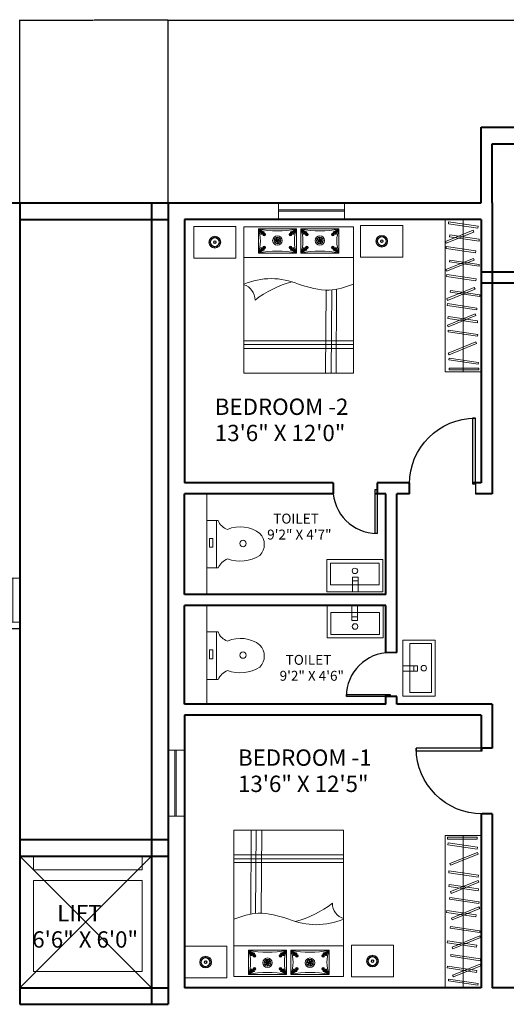
# Model space of a CAD drawing. Units: inches. Extents: x -46 to 1145, y -527 to 760.
# Tile 54 of 57: x 509 to 775, y 222 to 760. Entities that reach past the tile are written whole.
import ezdxf

# ---------------------------------------------------------------- set-up
doc = ezdxf.new("R2010")
doc.units = ezdxf.units.IN
doc.header["$MEASUREMENT"] = 0
for name, color, linetype, lineweight in [('A-ANNO-DIMS', 2, 'Continuous', 18), ('A-AREA-IDEN', 1, 'Continuous', 18), ('A-FLOR-CASE', 32, 'Continuous', 18), ('A-FLOR-EVTR', 6, 'Continuous', 18), ('A-FLOR-FIXT', 9, 'Continuous', 18), ('A-FURN', 2, 'Continuous', 13), ('DOORS', 3, 'Continuous', 25), ('WALLS', 4, 'Continuous', 40), ('WINDOWS', 240, 'Continuous', 20)]:
    doc.layers.add(name, color=color, linetype=linetype, lineweight=lineweight)
doc.layers.add('FURNTIURE', color=2, linetype='Continuous')
doc.layers.add('LT', color=9, linetype='Continuous')
doc.styles.get("Standard").update_dxf_attribs({"font": 'arial.ttf'})
doc.dimstyles.get("Standard").update_dxf_attribs({"dimtxt": 0.18, "dimasz": 0.18, "dimexe": 0.18, "dimexo": 0.0625, "dimgap": 0.09, "dimtad": 0, "dimtih": 1, "dimtoh": 1, "dimdec": 0, "dimzin": 0, "dimdsep": 46, "dimlunit": 3, "dimtxsty": 'Standard', "dimcen": 0.09, "dimadec": 0, "dimazin": 0, "dimtfac": 1, "dimtdec": 0, "dimtofl": 0, "dimtmove": 0, "dimatfit": 3, "dimfxl": 1, "dimtolj": 1, "dimtzin": 0, "dimarcsym": 0})

# ---------------------------------------------------------------- blocks, each defined once
blk = doc.blocks.new('*U2')
for p, q in [((0, 0), (0, -6)), ((40, 0), (40, -6))]:
    blk.add_line(p, q)
blk.add_lwpolyline([(0, 0), (0, 40), (1.75, 40), (1.75, 0)], close=True)
blk.add_arc((0, 0), 40, 0, 90)
blk = doc.blocks.new('*U89')
at = {"layer": 'FURNTIURE'}
blk.add_line((0, 0.42), (0, -0.42), dxfattribs=at)
blk = doc.blocks.new('*U90')
at = {"layer": 'FURNTIURE', "transparency": 16777216}
for p, rotation in [((589.5, 506.39), 54), ((590.11, 507), 36), ((590.89, 507.4), 17.99999999999997), ((592.61, 507.4), 341.9999999999999), ((593.39, 507), 324), ((594.01, 506.39), 306), ((588.97, 504.75), 90), ((589.1, 505.61), 72), ((589.1, 503.89), 108), ((589.5, 503.11), 126), ((590.11, 502.49), 144), ((590.89, 502.1), 162), ((591.75, 501.96), 180), ((592.61, 502.1), 197.9999999999999), ((593.39, 502.49), 216), ((594.01, 503.11), 234), ((594.4, 505.61), 288), ((594.4, 503.89), 252), ((594.54, 504.75), 270)]:
    blk.add_blockref('*U89', p, dxfattribs=dict(at, rotation=rotation))
blk.add_blockref('*U89', (591.75, 507.53), dxfattribs=at)
blk = doc.blocks.new('*U87')
at = {"layer": 'FURNTIURE'}
blk.add_line((0, 0.1), (0, -0.1), dxfattribs=at)
blk = doc.blocks.new('*U88')
at = {"layer": 'FURNTIURE', "transparency": 16777216}
for p, rotation in [((141.23, 121.04), 90), ((141.27, 121.25), 72), ((141.27, 120.83), 108), ((141.36, 121.43), 54), ((141.36, 120.65), 126), ((141.51, 121.58), 35.99999999999999), ((141.51, 120.5), 144), ((141.7, 121.67), 17.99999999999998), ((141.7, 120.4), 162), ((141.9, 120.37), 180), ((142.11, 121.67), 342), ((142.11, 120.4), 198), ((142.3, 121.58), 324), ((142.3, 120.5), 216), ((142.44, 121.43), 306), ((142.44, 120.65), 234), ((142.54, 121.25), 288), ((142.54, 120.83), 252), ((142.57, 121.04), 270)]:
    blk.add_blockref('*U87', p, dxfattribs=dict(at, rotation=rotation))
blk.add_blockref('*U87', (141.9, 121.71), dxfattribs=at)
blk = doc.blocks.new('NIGHTSTAND')
blk.add_lwpolyline([(23.06, 0), (0, 0), (0, 17.28), (23.06, 17.28)], close=True)
for radius in [3.21, 2.36, 0.77, 0.567]:
    blk.add_circle((11.53, 8.64), radius)
for name, p in [('*U90', (-580.22, -496.1)), ('*U88', (-130.37, -112.4))]:
    blk.add_blockref(name, p)
blk = doc.blocks.new('WARDROBE')
blk.add_line((9.78, 0), (9.78, 83.25))
for points in [[(19.56, 0), (0, 0), (0, 83.25), (19.56, 83.25)], [(17.74, 78.49), (1.66, 80.88), (1.8, 81.87), (17.88, 79.48)], [(15.55, 76.35), (0.49, 70.23), (0.11, 71.16), (15.17, 77.28)], [(18.43, 71.4), (2.35, 73.79), (2.5, 74.78), (18.58, 72.39)], [(16.47, 65.03), (0.39, 67.42), (0.54, 68.41), (16.62, 66.02)], [(15.79, 61), (0.73, 54.88), (0.35, 55.81), (15.41, 61.93)], [(18.43, 57.62), (2.35, 60.01), (2.5, 61), (18.58, 58.61)], [(16.71, 49.68), (0.63, 52.07), (0.78, 53.06), (16.86, 50.67)], [(16.22, 45.12), (1.16, 39), (0.78, 39.93), (15.84, 46.05)], [(18.77, 41.02), (2.69, 43.41), (2.84, 44.4), (18.92, 42.01)], [(17.14, 33.8), (1.06, 36.19), (1.21, 37.19), (17.29, 34.8)], [(16.65, 30.67), (1.59, 24.55), (1.21, 25.48), (16.27, 31.6)], [(17.52, 26.78), (1.44, 29.17), (1.59, 30.16), (17.67, 27.77)], [(17.57, 19.35), (1.49, 21.74), (1.64, 22.73), (17.72, 20.34)], [(17.08, 15.35), (2.02, 9.23), (1.64, 10.16), (16.7, 16.28)], [(18, 4.03), (1.92, 6.42), (2.07, 7.41), (18.15, 5.03)], [(18.32, 0.98), (2.07, 0.98), (2.07, 1.98), (18.32, 1.98)]]:
    blk.add_lwpolyline(points, close=True)
blk = doc.blocks.new('LAVATORY-RECT')
blk.add_line((14.01, 6.17), (17.08, 6.17))
for points in [[(30.61, 0), (0, 0), (0, 17.7), (30.61, 17.7)], [(28.7, 3.94), (1.97, 3.94), (1.97, 15.81), (28.7, 15.81)], [(17.08, 0), (14.01, 0), (14.01, 8.17), (17.08, 8.17)]]:
    blk.add_lwpolyline(points, close=True)
blk.add_circle((15.39, 11.51), 1.51)
blk = doc.blocks.new('WATER-CLOSET')
for p, q in [((0, 0), (0, 26.01)), ((0, 26.01), (6.13, 26.01)), ((5.22, 21.04), (5.22, 26.01)), ((5.22, 26.01), (5.22, 0)), ((0, 0), (6.13, 0))]:
    blk.add_line(p, q)
blk.add_lwpolyline([(1.51, 11.4), (1.51, 16.16), (3.34, 16.16), (3.34, 11.4)], close=True)
blk.add_circle((19.79, 13.37), 1.75)
for centre, radius, start, end in [((14.15, 29.2), 8.64, 201.6782, 251.0259), ((18.35, 4.96), 17.54, 52.4616, 113.5359), ((22.52, 12.84), 8.87, 317.2682, 42.7318), ((18.33, 23.71), 20, 249.5645, 302.3709), ((15.4, -4.5), 10.31, 113.1704, 154.0947)]:
    blk.add_arc(centre, radius, start, end)
blk = doc.blocks.new('WINDOW-36IN')
for p, q in [((0, 4.5), (0, 9)), ((0, 9), (0, 0)), ((36, 9), (36, 0)), ((0, 5.23), (36, 5.23)), ((0, 4.5), (36, 4.5))]:
    blk.add_line(p, q)
blk = doc.blocks.new('WINDOW-24IN')
for p, q in [((0, 4.5), (0, 9)), ((0, 9), (0, 0)), ((24, 9), (24, 0)), ((0, 5.23), (24, 5.23)), ((0, 4.5), (24, 4.5))]:
    blk.add_line(p, q)
blk = doc.blocks.new('*U58')
at = {"layer": 'LT'}
blk.add_line((0, 0.28), (0, -0.28), dxfattribs=at)
for centre, start, end in [((0.73, 0), 159.0676, 200.9324), ((-0.73, 0), 339.0676, 20.9324)]:
    blk.add_arc(centre, 0.786, start, end, dxfattribs=at)
blk = doc.blocks.new('*U59')
at = {"layer": 'LT', "transparency": 16777216}
for p, rotation in [((609.66, 443.79), 80.00000000000001), ((609.69, 443.6), 120), ((609.76, 443.96), 40.00000000000002), ((609.84, 443.48), 160), ((610.03, 443.48), 200), ((610.12, 443.96), 320), ((610.18, 443.6), 240), ((610.21, 443.79), 280)]:
    blk.add_blockref('*U58', p, dxfattribs=dict(at, rotation=rotation))
blk.add_blockref('*U58', (609.94, 444.03), dxfattribs=at)
blk = doc.blocks.new('*U60')
at = {"layer": 'LT'}
blk.add_line((0, 0.12), (0, -0.12), dxfattribs=at)
for centre, start, end in [((0.31, 0), 159.0676, 200.9324), ((-0.31, 0), 339.0676, 20.9324)]:
    blk.add_arc(centre, 0.335, start, end, dxfattribs=at)
blk = doc.blocks.new('*U61')
at = {"layer": 'LT', "transparency": 16777216}
for p, rotation in [((259.5, 188.9), 80.00000000000001), ((259.51, 188.82), 120), ((259.54, 188.97), 40), ((259.57, 188.76), 160), ((259.65, 188.76), 200), ((259.69, 188.97), 320), ((259.72, 188.82), 240), ((259.73, 188.9), 280)]:
    blk.add_blockref('*U60', p, dxfattribs=dict(at, rotation=rotation))
blk.add_blockref('*U60', (259.61, 189), dxfattribs=at)
blk = doc.blocks.new('*U62')
at = {"layer": 'LT'}
blk.add_line((0, 0.12), (0, -0.12), dxfattribs=at)
for centre, start, end in [((0.31, 0), 159.0676, 200.9324), ((-0.31, 0), 339.0676, 20.9324)]:
    blk.add_arc(centre, 0.335, start, end, dxfattribs=at)
blk = doc.blocks.new('*U63')
at = {"layer": 'LT', "transparency": 16777216}
for p, rotation in [((259.5, 188.9), 80.00000000000001), ((259.51, 188.82), 120), ((259.54, 188.97), 40), ((259.57, 188.76), 160), ((259.65, 188.76), 200), ((259.69, 188.97), 320), ((259.72, 188.82), 240), ((259.73, 188.9), 280)]:
    blk.add_blockref('*U62', p, dxfattribs=dict(at, rotation=rotation))
blk.add_blockref('*U62', (259.61, 189), dxfattribs=at)
blk = doc.blocks.new('*U64')
at = {"layer": 'LT'}
blk.add_line((0, 0.28), (0, -0.28), dxfattribs=at)
for centre, start, end in [((0.73, 0), 159.0676, 200.9324), ((-0.73, 0), 339.0676, 20.9324)]:
    blk.add_arc(centre, 0.786, start, end, dxfattribs=at)
blk = doc.blocks.new('*U65')
at = {"layer": 'LT', "transparency": 16777216}
for p, rotation in [((609.66, 443.79), 80.00000000000001), ((609.69, 443.6), 120), ((609.76, 443.96), 40.00000000000002), ((609.84, 443.48), 160), ((610.03, 443.48), 200), ((610.12, 443.96), 320), ((610.18, 443.6), 240), ((610.21, 443.79), 280)]:
    blk.add_blockref('*U64', p, dxfattribs=dict(at, rotation=rotation))
blk.add_blockref('*U64', (609.94, 444.03), dxfattribs=at)
blk = doc.blocks.new('*U66')
at = {"layer": 'LT'}
blk.add_line((0, 0.12), (0, -0.12), dxfattribs=at)
for centre, start, end in [((0.31, 0), 159.0676, 200.9324), ((-0.31, 0), 339.0676, 20.9324)]:
    blk.add_arc(centre, 0.335, start, end, dxfattribs=at)
blk = doc.blocks.new('*U67')
at = {"layer": 'LT', "transparency": 16777216}
for p, rotation in [((259.5, 188.9), 80.00000000000001), ((259.51, 188.82), 120), ((259.54, 188.97), 40), ((259.57, 188.76), 160), ((259.65, 188.76), 200), ((259.69, 188.97), 320), ((259.72, 188.82), 240), ((259.73, 188.9), 280)]:
    blk.add_blockref('*U66', p, dxfattribs=dict(at, rotation=rotation))
blk.add_blockref('*U66', (259.61, 189), dxfattribs=at)
blk = doc.blocks.new('*U68')
at = {"layer": 'LT'}
blk.add_line((0, 0.12), (0, -0.12), dxfattribs=at)
for centre, start, end in [((0.31, 0), 159.0676, 200.9324), ((-0.31, 0), 339.0676, 20.9324)]:
    blk.add_arc(centre, 0.335, start, end, dxfattribs=at)
blk = doc.blocks.new('*U69')
at = {"layer": 'LT', "transparency": 16777216}
for p, rotation in [((259.5, 188.9), 80.00000000000001), ((259.51, 188.82), 120), ((259.54, 188.97), 40), ((259.57, 188.76), 160), ((259.65, 188.76), 200), ((259.69, 188.97), 320), ((259.72, 188.82), 240), ((259.73, 188.9), 280)]:
    blk.add_blockref('*U68', p, dxfattribs=dict(at, rotation=rotation))
blk.add_blockref('*U68', (259.61, 189), dxfattribs=at)
blk = doc.blocks.new('*U70')
at = {"layer": 'LT'}
blk.add_line((0, 0.28), (0, -0.28), dxfattribs=at)
for centre, start, end in [((0.73, 0), 159.0676, 200.9324), ((-0.73, 0), 339.0676, 20.9324)]:
    blk.add_arc(centre, 0.786, start, end, dxfattribs=at)
blk = doc.blocks.new('*U71')
at = {"layer": 'LT', "transparency": 16777216}
for p, rotation in [((609.66, 443.79), 80.00000000000001), ((609.69, 443.6), 120), ((609.76, 443.96), 40.00000000000002), ((609.84, 443.48), 160), ((610.03, 443.48), 200), ((610.12, 443.96), 320), ((610.18, 443.6), 240), ((610.21, 443.79), 280)]:
    blk.add_blockref('*U70', p, dxfattribs=dict(at, rotation=rotation))
blk.add_blockref('*U70', (609.94, 444.03), dxfattribs=at)
blk = doc.blocks.new('*U46')
at = {"layer": 'LT'}
blk.add_line((0, 0.12), (0, -0.12), dxfattribs=at)
for centre, start, end in [((0.31, 0), 159.0676, 200.9324), ((-0.31, 0), 339.0676, 20.9324)]:
    blk.add_arc(centre, 0.335, start, end, dxfattribs=at)
blk = doc.blocks.new('*U47')
at = {"layer": 'LT', "transparency": 16777216}
for p, rotation in [((259.5, 188.9), 80.00000000000001), ((259.51, 188.82), 120), ((259.54, 188.97), 40), ((259.57, 188.76), 160), ((259.65, 188.76), 200), ((259.69, 188.97), 320), ((259.72, 188.82), 240), ((259.73, 188.9), 280)]:
    blk.add_blockref('*U46', p, dxfattribs=dict(at, rotation=rotation))
blk.add_blockref('*U46', (259.61, 189), dxfattribs=at)
blk = doc.blocks.new('*U48')
at = {"layer": 'LT'}
blk.add_line((0, 0.12), (0, -0.12), dxfattribs=at)
for centre, start, end in [((0.31, 0), 159.0676, 200.9324), ((-0.31, 0), 339.0676, 20.9324)]:
    blk.add_arc(centre, 0.335, start, end, dxfattribs=at)
blk = doc.blocks.new('*U49')
at = {"layer": 'LT', "transparency": 16777216}
for p, rotation in [((259.5, 188.9), 80.00000000000001), ((259.51, 188.82), 120), ((259.54, 188.97), 40), ((259.57, 188.76), 160), ((259.65, 188.76), 200), ((259.69, 188.97), 320), ((259.72, 188.82), 240), ((259.73, 188.9), 280)]:
    blk.add_blockref('*U48', p, dxfattribs=dict(at, rotation=rotation))
blk.add_blockref('*U48', (259.61, 189), dxfattribs=at)
blk = doc.blocks.new('*U50')
at = {"layer": 'LT'}
blk.add_line((0, 0.28), (0, -0.28), dxfattribs=at)
for centre, start, end in [((0.73, 0), 159.0676, 200.9324), ((-0.73, 0), 339.0676, 20.9324)]:
    blk.add_arc(centre, 0.786, start, end, dxfattribs=at)
blk = doc.blocks.new('*U51')
at = {"layer": 'LT', "transparency": 16777216}
for p, rotation in [((609.66, 443.79), 80.00000000000001), ((609.69, 443.6), 120), ((609.76, 443.96), 40.00000000000002), ((609.84, 443.48), 160), ((610.03, 443.48), 200), ((610.12, 443.96), 320), ((610.18, 443.6), 240), ((610.21, 443.79), 280)]:
    blk.add_blockref('*U50', p, dxfattribs=dict(at, rotation=rotation))
blk.add_blockref('*U50', (609.94, 444.03), dxfattribs=at)
blk = doc.blocks.new('*U52')
at = {"layer": 'LT'}
blk.add_line((0, 0.12), (0, -0.12), dxfattribs=at)
for centre, start, end in [((0.31, 0), 159.0676, 200.9324), ((-0.31, 0), 339.0676, 20.9324)]:
    blk.add_arc(centre, 0.335, start, end, dxfattribs=at)
blk = doc.blocks.new('*U53')
at = {"layer": 'LT', "transparency": 16777216}
for p, rotation in [((259.5, 188.9), 80.00000000000001), ((259.51, 188.82), 120), ((259.54, 188.97), 40), ((259.57, 188.76), 160), ((259.65, 188.76), 200), ((259.69, 188.97), 320), ((259.72, 188.82), 240), ((259.73, 188.9), 280)]:
    blk.add_blockref('*U52', p, dxfattribs=dict(at, rotation=rotation))
blk.add_blockref('*U52', (259.61, 189), dxfattribs=at)
blk = doc.blocks.new('*U54')
at = {"layer": 'LT'}
blk.add_line((0, 0.12), (0, -0.12), dxfattribs=at)
for centre, start, end in [((0.31, 0), 159.0676, 200.9324), ((-0.31, 0), 339.0676, 20.9324)]:
    blk.add_arc(centre, 0.335, start, end, dxfattribs=at)
blk = doc.blocks.new('*U55')
at = {"layer": 'LT', "transparency": 16777216}
for p, rotation in [((259.5, 188.9), 80.00000000000001), ((259.51, 188.82), 120), ((259.54, 188.97), 40), ((259.57, 188.76), 160), ((259.65, 188.76), 200), ((259.69, 188.97), 320), ((259.72, 188.82), 240), ((259.73, 188.9), 280)]:
    blk.add_blockref('*U54', p, dxfattribs=dict(at, rotation=rotation))
blk.add_blockref('*U54', (259.61, 189), dxfattribs=at)
blk = doc.blocks.new('*U34')
at = {"layer": 'LT'}
blk.add_line((0, 0.28), (0, -0.28), dxfattribs=at)
for centre, start, end in [((0.73, 0), 159.0676, 200.9324), ((-0.73, 0), 339.0676, 20.9324)]:
    blk.add_arc(centre, 0.786, start, end, dxfattribs=at)
blk = doc.blocks.new('*U35')
at = {"layer": 'LT', "transparency": 16777216}
for p, rotation in [((609.66, 443.79), 80.00000000000001), ((609.69, 443.6), 120), ((609.76, 443.96), 40.00000000000002), ((609.84, 443.48), 160), ((610.03, 443.48), 200), ((610.12, 443.96), 320), ((610.18, 443.6), 240), ((610.21, 443.79), 280)]:
    blk.add_blockref('*U34', p, dxfattribs=dict(at, rotation=rotation))
blk.add_blockref('*U34', (609.94, 444.03), dxfattribs=at)
blk = doc.blocks.new('*U36')
at = {"layer": 'LT'}
blk.add_line((0, 0.12), (0, -0.12), dxfattribs=at)
for centre, start, end in [((0.31, 0), 159.0676, 200.9324), ((-0.31, 0), 339.0676, 20.9324)]:
    blk.add_arc(centre, 0.335, start, end, dxfattribs=at)
blk = doc.blocks.new('*U37')
at = {"layer": 'LT', "transparency": 16777216}
for p, rotation in [((259.5, 188.9), 80.00000000000001), ((259.51, 188.82), 120), ((259.54, 188.97), 40), ((259.57, 188.76), 160), ((259.65, 188.76), 200), ((259.69, 188.97), 320), ((259.72, 188.82), 240), ((259.73, 188.9), 280)]:
    blk.add_blockref('*U36', p, dxfattribs=dict(at, rotation=rotation))
blk.add_blockref('*U36', (259.61, 189), dxfattribs=at)
blk = doc.blocks.new('*U38')
at = {"layer": 'LT'}
blk.add_line((0, 0.12), (0, -0.12), dxfattribs=at)
for centre, start, end in [((0.31, 0), 159.0676, 200.9324), ((-0.31, 0), 339.0676, 20.9324)]:
    blk.add_arc(centre, 0.335, start, end, dxfattribs=at)
blk = doc.blocks.new('*U39')
at = {"layer": 'LT', "transparency": 16777216}
for p, rotation in [((259.5, 188.9), 80.00000000000001), ((259.51, 188.82), 120), ((259.54, 188.97), 40), ((259.57, 188.76), 160), ((259.65, 188.76), 200), ((259.69, 188.97), 320), ((259.72, 188.82), 240), ((259.73, 188.9), 280)]:
    blk.add_blockref('*U38', p, dxfattribs=dict(at, rotation=rotation))
blk.add_blockref('*U38', (259.61, 189), dxfattribs=at)
blk = doc.blocks.new('*U40')
at = {"layer": 'LT'}
blk.add_line((0, 0.28), (0, -0.28), dxfattribs=at)
for centre, start, end in [((0.73, 0), 159.0676, 200.9324), ((-0.73, 0), 339.0676, 20.9324)]:
    blk.add_arc(centre, 0.786, start, end, dxfattribs=at)
blk = doc.blocks.new('*U41')
at = {"layer": 'LT', "transparency": 16777216}
for p, rotation in [((609.66, 443.79), 80.00000000000001), ((609.69, 443.6), 120), ((609.76, 443.96), 40.00000000000002), ((609.84, 443.48), 160), ((610.03, 443.48), 200), ((610.12, 443.96), 320), ((610.18, 443.6), 240), ((610.21, 443.79), 280)]:
    blk.add_blockref('*U40', p, dxfattribs=dict(at, rotation=rotation))
blk.add_blockref('*U40', (609.94, 444.03), dxfattribs=at)
blk = doc.blocks.new('*U42')
at = {"layer": 'LT'}
blk.add_line((0, 0.12), (0, -0.12), dxfattribs=at)
for centre, start, end in [((0.31, 0), 159.0676, 200.9324), ((-0.31, 0), 339.0676, 20.9324)]:
    blk.add_arc(centre, 0.335, start, end, dxfattribs=at)
blk = doc.blocks.new('*U43')
at = {"layer": 'LT', "transparency": 16777216}
for p, rotation in [((259.5, 188.9), 80.00000000000001), ((259.51, 188.82), 120), ((259.54, 188.97), 40), ((259.57, 188.76), 160), ((259.65, 188.76), 200), ((259.69, 188.97), 320), ((259.72, 188.82), 240), ((259.73, 188.9), 280)]:
    blk.add_blockref('*U42', p, dxfattribs=dict(at, rotation=rotation))
blk.add_blockref('*U42', (259.61, 189), dxfattribs=at)
blk = doc.blocks.new('*U44')
at = {"layer": 'LT'}
blk.add_line((0, 0.12), (0, -0.12), dxfattribs=at)
for centre, start, end in [((0.31, 0), 159.0676, 200.9324), ((-0.31, 0), 339.0676, 20.9324)]:
    blk.add_arc(centre, 0.335, start, end, dxfattribs=at)
blk = doc.blocks.new('*U45')
at = {"layer": 'LT', "transparency": 16777216}
for p, rotation in [((259.5, 188.9), 80.00000000000001), ((259.51, 188.82), 120), ((259.54, 188.97), 40), ((259.57, 188.76), 160), ((259.65, 188.76), 200), ((259.69, 188.97), 320), ((259.72, 188.82), 240), ((259.73, 188.9), 280)]:
    blk.add_blockref('*U44', p, dxfattribs=dict(at, rotation=rotation))
blk.add_blockref('*U44', (259.61, 189), dxfattribs=at)
blk = doc.blocks.new('*U72')
at = {"layer": 'LT'}
blk.add_line((0, 0.28), (0, -0.28), dxfattribs=at)
for centre, start, end in [((0.73, 0), 159.0676, 200.9324), ((-0.73, 0), 339.0676, 20.9324)]:
    blk.add_arc(centre, 0.786, start, end, dxfattribs=at)
blk = doc.blocks.new('*U73')
at = {"layer": 'LT', "transparency": 16777216}
for p, rotation in [((609.66, 443.79), 80.00000000000001), ((609.69, 443.6), 120), ((609.76, 443.96), 40.00000000000002), ((609.84, 443.48), 160), ((610.03, 443.48), 200), ((610.12, 443.96), 320), ((610.18, 443.6), 240), ((610.21, 443.79), 280)]:
    blk.add_blockref('*U72', p, dxfattribs=dict(at, rotation=rotation))
blk.add_blockref('*U72', (609.94, 444.03), dxfattribs=at)
blk = doc.blocks.new('*U74')
at = {"layer": 'LT'}
blk.add_line((0, 0.12), (0, -0.12), dxfattribs=at)
for centre, start, end in [((0.31, 0), 159.0676, 200.9324), ((-0.31, 0), 339.0676, 20.9324)]:
    blk.add_arc(centre, 0.335, start, end, dxfattribs=at)
blk = doc.blocks.new('*U75')
at = {"layer": 'LT', "transparency": 16777216}
for p, rotation in [((259.5, 188.9), 80.00000000000001), ((259.51, 188.82), 120), ((259.54, 188.97), 40), ((259.57, 188.76), 160), ((259.65, 188.76), 200), ((259.69, 188.97), 320), ((259.72, 188.82), 240), ((259.73, 188.9), 280)]:
    blk.add_blockref('*U74', p, dxfattribs=dict(at, rotation=rotation))
blk.add_blockref('*U74', (259.61, 189), dxfattribs=at)
blk = doc.blocks.new('*U76')
at = {"layer": 'LT'}
blk.add_line((0, 0.12), (0, -0.12), dxfattribs=at)
for centre, start, end in [((0.31, 0), 159.0676, 200.9324), ((-0.31, 0), 339.0676, 20.9324)]:
    blk.add_arc(centre, 0.335, start, end, dxfattribs=at)
blk = doc.blocks.new('*U77')
at = {"layer": 'LT', "transparency": 16777216}
for p, rotation in [((259.5, 188.9), 80.00000000000001), ((259.51, 188.82), 120), ((259.54, 188.97), 40), ((259.57, 188.76), 160), ((259.65, 188.76), 200), ((259.69, 188.97), 320), ((259.72, 188.82), 240), ((259.73, 188.9), 280)]:
    blk.add_blockref('*U76', p, dxfattribs=dict(at, rotation=rotation))
blk.add_blockref('*U76', (259.61, 189), dxfattribs=at)
blk = doc.blocks.new('*U78')
at = {"layer": 'LT'}
blk.add_line((0, 0.28), (0, -0.28), dxfattribs=at)
for centre, start, end in [((0.73, 0), 159.0676, 200.9324), ((-0.73, 0), 339.0676, 20.9324)]:
    blk.add_arc(centre, 0.786, start, end, dxfattribs=at)
blk = doc.blocks.new('*U79')
at = {"layer": 'LT', "transparency": 16777216}
for p, rotation in [((609.66, 443.79), 80.00000000000001), ((609.69, 443.6), 120), ((609.76, 443.96), 40.00000000000002), ((609.84, 443.48), 160), ((610.03, 443.48), 200), ((610.12, 443.96), 320), ((610.18, 443.6), 240), ((610.21, 443.79), 280)]:
    blk.add_blockref('*U78', p, dxfattribs=dict(at, rotation=rotation))
blk.add_blockref('*U78', (609.94, 444.03), dxfattribs=at)
blk = doc.blocks.new('*U80')
at = {"layer": 'LT'}
blk.add_line((0, 0.12), (0, -0.12), dxfattribs=at)
for centre, start, end in [((0.31, 0), 159.0676, 200.9324), ((-0.31, 0), 339.0676, 20.9324)]:
    blk.add_arc(centre, 0.335, start, end, dxfattribs=at)
blk = doc.blocks.new('*U81')
at = {"layer": 'LT', "transparency": 16777216}
for p, rotation in [((259.5, 188.9), 80.00000000000001), ((259.51, 188.82), 120), ((259.54, 188.97), 40), ((259.57, 188.76), 160), ((259.65, 188.76), 200), ((259.69, 188.97), 320), ((259.72, 188.82), 240), ((259.73, 188.9), 280)]:
    blk.add_blockref('*U80', p, dxfattribs=dict(at, rotation=rotation))
blk.add_blockref('*U80', (259.61, 189), dxfattribs=at)
blk = doc.blocks.new('*U82')
at = {"layer": 'LT'}
blk.add_line((0, 0.12), (0, -0.12), dxfattribs=at)
for centre, start, end in [((0.31, 0), 159.0676, 200.9324), ((-0.31, 0), 339.0676, 20.9324)]:
    blk.add_arc(centre, 0.335, start, end, dxfattribs=at)
blk = doc.blocks.new('*U83')
at = {"layer": 'LT', "transparency": 16777216}
for p, rotation in [((259.5, 188.9), 80.00000000000001), ((259.51, 188.82), 120), ((259.54, 188.97), 40), ((259.57, 188.76), 160), ((259.65, 188.76), 200), ((259.69, 188.97), 320), ((259.72, 188.82), 240), ((259.73, 188.9), 280)]:
    blk.add_blockref('*U82', p, dxfattribs=dict(at, rotation=rotation))
blk.add_blockref('*U82', (259.61, 189), dxfattribs=at)
blk = doc.blocks.new('*U32')
at = {"layer": 'FURNTIURE'}
blk.add_open_spline([(0.04, 1.82), (-0.22, 1.45), (-0.66, 0.8), (0.1, -0.02), (0.64, -0.93), (0.24, -1.53), (0.04, -1.82)], degree=3, knots=[0, 0, 0, 0, 1.177175, 2.037162, 3.056205, 4.032246, 4.032246, 4.032246, 4.032246], dxfattribs=at)
blk = doc.blocks.new('*U33')
at = {"layer": 'FURNTIURE', "transparency": 16777216}
for p, rotation in [((904.32, 663.42), 300), ((904.32, 663.35), 59.99999999999999), ((904.36, 663.42), 239.9999999999999), ((904.36, 663.35), 119.9999999999999), ((904.38, 663.38), 180)]:
    blk.add_blockref('*U32', p, dxfattribs=dict(at, rotation=rotation))
blk.add_blockref('*U32', (904.3, 663.38), dxfattribs=at)
blk = doc.blocks.new('*U56')
at = {"layer": 'FURNTIURE'}
blk.add_open_spline([(0.04, 1.82), (-0.22, 1.45), (-0.66, 0.8), (0.1, -0.02), (0.64, -0.93), (0.24, -1.53), (0.04, -1.82)], degree=3, knots=[0, 0, 0, 0, 1.177175, 2.037162, 3.056205, 4.032246, 4.032246, 4.032246, 4.032246], dxfattribs=at)
blk = doc.blocks.new('*U57')
at = {"layer": 'FURNTIURE', "transparency": 16777216}
for p, rotation in [((904.32, 663.42), 300), ((904.32, 663.35), 59.99999999999999), ((904.36, 663.42), 239.9999999999999), ((904.36, 663.35), 119.9999999999999), ((904.38, 663.38), 180)]:
    blk.add_blockref('*U56', p, dxfattribs=dict(at, rotation=rotation))
blk.add_blockref('*U56', (904.3, 663.38), dxfattribs=at)
blk = doc.blocks.new('BED-QUEEN-FURNISHED')
for p, q in [((0, 0), (0, 80)), ((0, 80), (60, 80)), ((8, 78.8), (28.8, 78.8)), ((8, 65.6), (8, 78.8)), ((8, 78.8), (11.38, 75.61)), ((8, 78.8), (9.68, 76.18)), ((8, 78.8), (10.93, 76.98)), ((10.93, 76.98), (10.93, 76.75)), ((11.25, 75.74), (11.25, 75.18)), ((28.8, 78.8), (25.41, 75.61)), ((25.55, 75.74), (25.55, 75.18)), ((28.8, 78.8), (25.87, 76.98)), ((25.87, 76.98), (25.87, 76.75)), ((28.8, 78.8), (27.12, 76.18)), ((27.12, 76.18), (27.12, 75.95)), ((28.8, 78.8), (28.8, 65.6)), ((31.2, 78.8), (52, 78.8)), ((31.2, 65.6), (31.2, 78.8)), ((31.2, 78.8), (52, 78.8)), ((31.2, 65.6), (31.2, 78.8)), ((31.2, 78.8), (34.58, 75.61)), ((31.2, 78.8), (32.88, 76.18)), ((31.2, 78.8), (34.13, 76.98)), ((34.13, 76.98), (34.13, 76.75)), ((34.45, 75.74), (34.45, 75.18)), ((52, 78.8), (48.61, 75.61)), ((48.75, 75.74), (48.75, 75.18)), ((52, 78.8), (49.07, 76.98)), ((49.07, 76.98), (49.07, 76.75)), ((52, 78.8), (50.32, 76.18)), ((50.32, 76.18), (50.32, 75.95)), ((52, 78.8), (52, 65.6)), ((52, 78.8), (52, 65.6)), ((60, 80), (60, 0)), ((8, 65.61), (11.38, 68.8)), ((8, 65.61), (9.68, 68.23)), ((8, 65.61), (10.92, 67.43)), ((8, 65.6), (28.8, 65.6)), ((10.92, 67.43), (10.92, 67.67)), ((11.25, 68.67), (11.25, 69.23)), ((28.8, 65.6), (25.41, 68.79)), ((25.87, 67.42), (25.87, 67.66)), ((28.8, 65.6), (25.87, 67.42)), ((27.11, 68.22), (27.11, 68.46)), ((28.8, 65.6), (27.11, 68.22)), ((31.2, 65.61), (34.58, 68.8)), ((31.2, 65.61), (32.88, 68.23)), ((31.2, 65.61), (34.12, 67.43)), ((31.2, 65.6), (52, 65.6)), ((31.2, 65.6), (52, 65.6)), ((34.12, 67.43), (34.12, 67.67)), ((34.45, 68.67), (34.45, 69.23)), ((52, 65.6), (48.61, 68.79)), ((49.07, 67.42), (49.07, 67.66)), ((52, 65.6), (49.07, 67.42)), ((50.31, 68.22), (50.31, 68.46)), ((52, 65.6), (50.31, 68.22)), ((60, 63.2), (0, 63.2)), ((46.8, 63.6), (46.8, 63.6)), ((44.72, 0), (45.02, 45.37)), ((47.8, 0), (48.1, 45.5)), ((50.46, 0), (50.76, 45.91)), ((0, 17.7), (60, 17.7)), ((0, 15.69), (60, 15.69)), ((0, 13.42), (60, 13.42)), ((60, 0), (0, 0))]:
    blk.add_line(p, q)
for centre, radius in [((9.68, 76.18), 0.308), ((9.68, 76.18), 0.239), ((11.25, 75.74), 0.723), ((10.93, 76.98), 0.308), ((10.93, 76.98), 0.239), ((11.25, 75.74), 0.562), ((25.55, 75.74), 0.723), ((25.55, 75.74), 0.562), ((25.87, 76.98), 0.308), ((25.87, 76.98), 0.239), ((27.12, 76.18), 0.308), ((27.12, 76.18), 0.239), ((32.88, 76.18), 0.308), ((32.88, 76.18), 0.239), ((34.45, 75.74), 0.723), ((34.13, 76.98), 0.308), ((34.13, 76.98), 0.239), ((34.45, 75.74), 0.562), ((48.75, 75.74), 0.723), ((48.75, 75.74), 0.562), ((49.07, 76.98), 0.308), ((49.07, 76.98), 0.239), ((50.32, 76.18), 0.308), ((50.32, 76.18), 0.239), ((18.4, 72.44), 2.6), ((18.4, 72.44), 1.82), ((41.6, 72.44), 2.6), ((41.6, 72.44), 1.82), ((9.68, 68.23), 0.308), ((9.68, 68.23), 0.239), ((11.25, 68.67), 0.723), ((10.92, 67.43), 0.308), ((10.92, 67.43), 0.239), ((11.25, 68.67), 0.562), ((25.55, 68.66), 0.723), ((25.55, 68.66), 0.562), ((25.87, 67.42), 0.308), ((25.87, 67.42), 0.239), ((27.11, 68.22), 0.308), ((27.11, 68.22), 0.239), ((32.88, 68.23), 0.308), ((32.88, 68.23), 0.239), ((34.45, 68.67), 0.723), ((34.12, 67.43), 0.308), ((34.12, 67.43), 0.239), ((34.45, 68.67), 0.562), ((48.75, 68.66), 0.723), ((48.75, 68.66), 0.562), ((49.07, 67.42), 0.308), ((49.07, 67.42), 0.239), ((50.31, 68.22), 0.308), ((50.31, 68.22), 0.239)]:
    blk.add_circle(centre, radius)
for centre, radius, start, end in [((18.4, 129.18), 51.44, 258.3356, 281.6644), ((-10.65, 72.2), 19.79, 340.5151, 19.4849), ((11.24, 76.86), 0.335, 159.0676, 200.9324), ((10.61, 76.86), 0.335, 339.0676, 20.9324), ((11.99, 75.46), 0.786, 159.0676, 200.9324), ((10.52, 75.46), 0.786, 339.0676, 20.9324), ((26.28, 75.46), 0.786, 159.0676, 200.9324), ((24.81, 75.46), 0.786, 339.0676, 20.9324), ((26.19, 76.86), 0.335, 159.0676, 200.9324), ((25.56, 76.86), 0.335, 339.0676, 20.9324), ((27.43, 76.06), 0.335, 159.0676, 200.9324), ((26.8, 76.06), 0.335, 339.0676, 20.9324), ((47.45, 72.2), 19.79, 160.5151, 199.4849), ((41.6, 129.18), 51.44, 258.3356, 281.6644), ((12.55, 72.2), 19.79, 340.5151, 19.4849), ((34.44, 76.86), 0.335, 159.0676, 200.9324), ((33.81, 76.86), 0.335, 339.0676, 20.9324), ((35.19, 75.46), 0.786, 159.0676, 200.9324), ((33.72, 75.46), 0.786, 339.0676, 20.9324), ((49.48, 75.46), 0.786, 159.0676, 200.9324), ((48.01, 75.46), 0.786, 339.0676, 20.9324), ((49.39, 76.86), 0.335, 159.0676, 200.9324), ((48.76, 76.86), 0.335, 339.0676, 20.9324), ((50.63, 76.06), 0.335, 159.0676, 200.9324), ((50, 76.06), 0.335, 339.0676, 20.9324), ((70.65, 72.2), 19.79, 160.5151, 199.4849), ((18.4, 15.22), 51.44, 78.3356, 101.6644), ((11.24, 67.55), 0.335, 159.028, 200.8928), ((10.61, 67.55), 0.335, 339.028, 20.8928), ((11.98, 68.95), 0.786, 159.028, 200.8928), ((10.51, 68.95), 0.786, 339.028, 20.8928), ((26.18, 67.54), 0.335, 159.028, 200.8928), ((25.56, 67.54), 0.335, 339.028, 20.8928), ((27.43, 68.34), 0.335, 159.028, 200.8928), ((26.8, 68.34), 0.335, 339.028, 20.8928), ((41.6, 15.22), 51.44, 78.3356, 101.6644), ((34.44, 67.55), 0.335, 159.028, 200.8928), ((33.81, 67.55), 0.335, 339.028, 20.8928), ((35.18, 68.95), 0.786, 159.028, 200.8928), ((33.71, 68.95), 0.786, 339.028, 20.8928), ((49.38, 67.54), 0.335, 159.028, 200.8928), ((48.76, 67.54), 0.335, 339.028, 20.8928), ((50.63, 68.34), 0.335, 159.028, 200.8928), ((50, 68.34), 0.335, 339.028, 20.8928), ((15, 13.08), 38.56, 67.1089, 112.8911), ((40.88, -5.13), 56.88, 104.6834, 127.6009), ((40.88, -5.13), 56.88, 70.3635, 70.606), ((-2.62, 39.94), 8.8, 0, 72.6522)]:
    blk.add_arc(centre, radius, start, end)
blk.add_open_spline([(30, 48.6), (35.57, 46.87), (45.64, 43.74), (55.56, 47.1), (60, 48.6)], degree=3, knots=[0, 0, 0, 0, 16.971495, 30.687365, 30.687365, 30.687365, 30.687365])
at = {"xscale": -1}
for name, p in [('*U43', (269.3, -112.69)), ('*U45', (270.54, -111.89)), ('*U41', (621.19, -368.01)), ('*U67', (292.5, -112.69)), ('*U69', (293.74, -111.89)), ('*U65', (644.39, -368.01))]:
    blk.add_blockref(name, p, dxfattribs=at)
for name, p in [('*U35', (-584.39, -368.01)), ('*U39', (-233.74, -111.89)), ('*U37', (-232.5, -112.69)), ('*U59', (-561.19, -368.01)), ('*U63', (-210.54, -111.89)), ('*U61', (-209.3, -112.69)), ('*U33', (-885.94, -590.95)), ('*U57', (-862.74, -590.95))]:
    blk.add_blockref(name, p)
at = {"rotation": 179.9603994254766}
for name, p in [('*U81', (269.43, 256.92)), ('*U83', (270.67, 256.12)), ('*U79', (621.49, 512)), ('*U53', (292.63, 256.92)), ('*U55', (293.87, 256.12)), ('*U51', (644.69, 512))]:
    blk.add_blockref(name, p, dxfattribs=at)
at = {"xscale": -1, "rotation": 179.9603994254766}
for name, p in [('*U73', (-584.08, 512.83)), ('*U77', (-233.61, 256.47)), ('*U75', (-232.37, 257.27)), ('*U71', (-560.88, 512.83)), ('*U49', (-210.41, 256.47)), ('*U47', (-209.17, 257.27))]:
    blk.add_blockref(name, p, dxfattribs=at)
blk = doc.blocks.new('*D665')
at = {"layer": 'A-ANNO-DIMS', "color": 0, "lineweight": -2, "transparency": 16777216}
for p, q in [((500.06, 430.36), (500.06, 426.64)), ((500.24, 426.82), (504.11, 426.82)), ((508.88, 426.82), (505.02, 426.82)), ((509.06, 430.36), (509.06, 426.64))]:
    blk.add_line(p, q, dxfattribs=at)
at = {"layer": 'A-ANNO-DIMS', "color": 0, "transparency": 16777216}
for points in [[(500.24, 426.85), (500.24, 426.79), (500.06, 426.82)], [(508.88, 426.85), (508.88, 426.79), (509.06, 426.82)]]:
    blk.add_solid(points, dxfattribs=at)
at = {"layer": 'Defpoints', "color": 0, "transparency": 16777216}
for p in [(500.06, 430.42), (509.06, 430.42), (509.06, 426.82)]:
    blk.add_point(p, dxfattribs=at)
at = {"layer": 'A-ANNO-DIMS', "color": 0, "transparency": 16777216, "insert": (504.56, 426.82), "char_height": 0.18, "attachment_point": 5}
blk.add_mtext('\\A1;9 TYP.', dxfattribs=at)
blk = doc.blocks.new('*D686')
at = {"layer": 'A-ANNO-DIMS', "color": 0, "lineweight": -2, "transparency": 16777216}
for p, q in [((590.06, 659.58), (590.06, 759.67)), ((590.24, 759.49), (837.92, 759.49)), ((1086.38, 759.49), (838.71, 759.49)), ((1086.56, 659.58), (1086.56, 759.67))]:
    blk.add_line(p, q, dxfattribs=at)
at = {"layer": 'A-ANNO-DIMS', "color": 0, "transparency": 16777216}
for points in [[(590.24, 759.52), (590.24, 759.46), (590.06, 759.49)], [(1086.38, 759.52), (1086.38, 759.46), (1086.56, 759.49)]]:
    blk.add_solid(points, dxfattribs=at)
at = {"layer": 'Defpoints', "color": 0, "transparency": 16777216}
for p in [(1086.56, 759.49), (590.06, 659.52), (1086.56, 659.52)]:
    blk.add_point(p, dxfattribs=at)
at = {"layer": 'A-ANNO-DIMS', "color": 0, "transparency": 16777216, "insert": (838.31, 759.49), "char_height": 0.18, "attachment_point": 5}
blk.add_mtext('\\A1;496.5', dxfattribs=at)
blk = doc.blocks.new('*D687')
at = {"layer": 'A-ANNO-DIMS', "color": 0, "lineweight": -2, "transparency": 16777216}
for p, q in [((509.06, 659.58), (509.06, 759.67)), ((509.24, 759.49), (549.36, 759.49)), ((589.88, 759.49), (549.77, 759.49)), ((590.06, 659.58), (590.06, 759.67))]:
    blk.add_line(p, q, dxfattribs=at)
at = {"layer": 'A-ANNO-DIMS', "color": 0, "transparency": 16777216}
for points in [[(509.24, 759.52), (509.24, 759.46), (509.06, 759.49)], [(589.88, 759.52), (589.88, 759.46), (590.06, 759.49)]]:
    blk.add_solid(points, dxfattribs=at)
at = {"layer": 'Defpoints', "color": 0, "transparency": 16777216}
for p in [(590.06, 759.49), (509.06, 659.52), (590.06, 659.52)]:
    blk.add_point(p, dxfattribs=at)
at = {"layer": 'A-ANNO-DIMS', "color": 0, "transparency": 16777216, "insert": (549.56, 759.49), "char_height": 0.18, "attachment_point": 5}
blk.add_mtext('\\A1;81', dxfattribs=at)

msp = doc.modelspace()

# ---------------------------------------------------------------- linework, layer by layer
at = {"layer": 'A-FLOR-CASE'}
for p, q in [((611.2427, 500.5176), (611.2427, 445.5176)), ((611.2427, 439.5176), (611.2427, 385.5176))]:
    msp.add_line(p, q, dxfattribs=at)
at = {"layer": 'A-FLOR-EVTR'}
for p, q in [((509.0637, 230.5176), (581.0637, 302.5176)), ((581.0637, 230.5176), (509.0637, 302.5176))]:
    msp.add_line(p, q, dxfattribs=at)
for points in [[(516.5658, 302.5176), (575.899, 302.5176), (575.899, 294.9554), (516.5658, 294.9554)], [(575.899, 239.4948), (516.5658, 239.4948), (516.5658, 289.1419), (575.899, 289.1419)]]:
    msp.add_lwpolyline(points, close=True, dxfattribs=at)
at = {"layer": 'WALLS'}
for p, q in [((761.0637, 659.5176), (761.0637, 700.8886)), ((761.0637, 700.8886), (767.0637, 700.8886)), ((767.0637, 700.8886), (917.0637, 700.8886)), ((767.0637, 691.8886), (911.0637, 691.8886)), ((767.0637, 659.5176), (767.0637, 691.8886)), ((339.5637, 659.5176), (509.0637, 659.5176)), ((509.0637, 659.5176), (509.0637, 221.5176)), ((509.0637, 659.5176), (590.0637, 659.5176)), ((581.0637, 659.5176), (581.0637, 221.5176)), ((590.0637, 659.5176), (590.0637, 221.5176)), ((590.0637, 659.5176), (590.0637, 221.5176)), ((590.0637, 659.5176), (761.0637, 659.5176)), ((767.0637, 659.5176), (767.0637, 500.5176)), ((509.0637, 650.5176), (590.0637, 650.5176)), ((599.0637, 650.5176), (599.0637, 506.5176)), ((761.0637, 650.5176), (599.0637, 650.5176)), ((761.0637, 650.5176), (761.0637, 506.5176)), ((761.0637, 621.8886), (911.0637, 621.8886)), ((761.0637, 615.8886), (911.0637, 615.8886)), ((680.2169, 506.5176), (599.0637, 506.5176)), ((680.2169, 506.5176), (680.3372, 500.5176)), ((721.9431, 506.5176), (704.2169, 506.5176)), ((704.2169, 506.5176), (704.2169, 500.5176)), ((721.9381, 500.5176), (721.9381, 506.5176)), ((761.0637, 506.5176), (756.3631, 506.5176)), ((757.9381, 505.9176), (757.9381, 506.5176)), ((680.3372, 500.5176), (599.0637, 500.5176)), ((599.0637, 445.5176), (599.0637, 500.5176)), ((709.0637, 500.5176), (703.1669, 500.5176)), ((709.0637, 445.5176), (709.0637, 500.5176)), ((721.9381, 500.5176), (715.0637, 500.5176)), ((715.0637, 439.5176), (715.0637, 500.5176)), ((767.0637, 500.5176), (757.9381, 500.5176)), ((709.0637, 445.5176), (599.0637, 445.5176)), ((709.0637, 439.5176), (599.0637, 439.5176)), ((599.0637, 385.5176), (599.0637, 439.5176)), ((709.0637, 413.6562), (709.0637, 439.5176)), ((715.0637, 413.7765), (715.0637, 439.5176)), ((715.0637, 413.7765), (709.0637, 413.6562)), ((709.0637, 385.5176), (709.0637, 390.8265)), ((715.0637, 389.7765), (709.0637, 389.7765)), ((715.0637, 385.5176), (715.0637, 389.7765)), ((709.0637, 385.5176), (599.0637, 385.5176)), ((767.0637, 385.5176), (715.0637, 385.5176)), ((767.0637, 385.5176), (767.0637, 361.5613)), ((599.0637, 379.5176), (599.0637, 230.5176)), ((761.0637, 379.5176), (599.0637, 379.5176)), ((761.0637, 379.5176), (761.0637, 359.9863)), ((767.0637, 361.5613), (761.0637, 361.5613)), ((761.0637, 325.5663), (761.0637, 230.5176)), ((767.0637, 325.5613), (761.6637, 325.5613)), ((767.0637, 325.5613), (767.0637, 230.5176)), ((509.0637, 311.5176), (590.0637, 311.5176)), ((509.0637, 302.5176), (590.0637, 302.5176)), ((509.0637, 230.5176), (590.0637, 230.5176)), ((761.0637, 230.5176), (599.0637, 230.5176)), ((787.3481, 230.5176), (767.0637, 230.5176)), ((509.0637, 221.5176), (590.0637, 221.5176))]:
    msp.add_line(p, q, dxfattribs=at)

# ---------------------------------------------------------------- block references
at = {"layer": 'A-FLOR-CASE'}
msp.add_blockref('WARDROBE', (741.504, 567.272), dxfattribs=at)
at = {"layer": 'A-FLOR-CASE', "rotation": 180}
msp.add_blockref('WARDROBE', (761.0642, 313.7631), dxfattribs=at)
at = {"layer": 'A-FLOR-FIXT'}
for name, p in [('WATER-CLOSET', (611.243, 460.011)), ('LAVATORY-RECT', (676.752, 446.889)), ('WATER-CLOSET', (611.243, 399.011))]:
    msp.add_blockref(name, p, dxfattribs=at)
for p, rotation in [((707.611, 439.5176), 180), ((718.2357, 420.605), 269.9999999999989)]:
    msp.add_blockref('LAVATORY-RECT', p, dxfattribs=dict(at, rotation=rotation))
at = {"layer": 'A-FURN'}
for name, p in [('NIGHTSTAND', (604.126, 629.415)), ('BED-QUEEN-FURNISHED', (631.41, 566.503)), ('NIGHTSTAND', (695.2733, 629.954))]:
    msp.add_blockref(name, p, dxfattribs=at)
at = {"layer": 'A-FURN', "rotation": 180}
for name, p in [('BED-QUEEN-FURNISHED', (685.9877, 316.6818)), ('NIGHTSTAND', (622.1243, 253.2307)), ('NIGHTSTAND', (713.2717, 253.7698))]:
    msp.add_blockref(name, p, dxfattribs=at)
at = {"layer": 'DOORS', "xscale": -0.9, "yscale": 0.9, "zscale": 0.9}
msp.add_blockref('*U2', (757.9381, 505.9176), dxfattribs=at)
at = {"layer": 'DOORS'}
for p, xscale, yscale, zscale, rotation in [((704.2169, 502.9176), 0.6, 0.6, 0.6, 180), ((711.4637, 389.7765), 0.6, 0.6, 0.6, 90), ((761.6637, 361.5613), -0.9, 0.9, 0.9, 90)]:
    msp.add_blockref('*U2', p, dxfattribs=dict(at, xscale=xscale, yscale=yscale, zscale=zscale, rotation=rotation))
at = {"layer": 'WINDOWS'}
msp.add_blockref('WINDOW-36IN', (650.495, 650.518), dxfattribs=at)
for name, p, rotation in [('WINDOW-24IN', (500.0642, 454.4195), 270.0000000000003), ('WINDOW-36IN', (599.0633, 324.3306), 89.99999999999976)]:
    msp.add_blockref(name, p, dxfattribs=dict(at, rotation=rotation))

# ---------------------------------------------------------------- texts
at = {"layer": 'A-AREA-IDEN'}
for s, height, p in [('BEDROOM -2 ', 8.923264, (615.6454, 543.6508)), ('13\'6" X 12\'0"', 8.923264, (615.6454, 529.3164)), ('   TOILET', 5.42821, (642.5585, 484.264)), (' 9\'2" X 4\'7"', 5.428214, (642.5585, 475.544)), ('   TOILET', 5.42821, (649.3549, 407.0717)), (' 9\'2" X 4\'6"', 5.428214, (649.3549, 398.3518)), ('BEDROOM -1 ', 8.923264, (628.3065, 351.892)), ('13\'6" X 12\'5"', 8.923264, (628.3065, 337.5576)), ('     LIFT', 8.92326, (515.9197, 266.8323)), ('6\'6" X 6\'0"', 8.923264, (515.9197, 252.4979))]:
    msp.add_text(s, height=height, dxfattribs=at).set_placement(p)

# ---------------------------------------------------------------- dimensions: what is measured, and where the dimension line sits
at = {"layer": 'A-ANNO-DIMS'}
for base, p1, p2, override, picture, middle in [((590.0637, 759.4886), (509.0637, 659.5176), (590.0637, 659.5176), {"dimdec": 0, "dimlfac": 1, "dimrnd": 0, "dimzin": 0, "dimdsep": 46, "dimlunit": 2}, '*D687', (549.5637, 759.4886)), ((1086.5637, 759.4886), (590.0637, 659.5176), (1086.5637, 659.5176), {"dimdec": 1, "dimlfac": 1, "dimrnd": 0, "dimzin": 0, "dimdsep": 46, "dimlunit": 2}, '*D686', (838.3137, 759.4886))]:
    dim = msp.add_linear_dim(base=base, p1=p1, p2=p2, dimstyle='Standard', override=override, dxfattribs=at)
    dim.commit()
    dim.dimension.update_dxf_attribs({"geometry": picture, "text_midpoint": middle})
dim = msp.add_linear_dim(base=(509.0637, 426.8192), p1=(500.0637, 430.4192), p2=(509.0637, 430.4192), angle=0, text='<> TYP.', dimstyle='Standard', override={"dimdec": 0, "dimlfac": 1, "dimrnd": 0, "dimzin": 0, "dimdsep": 46, "dimlunit": 2}, dxfattribs=at)
dim.commit()
dim.dimension.update_dxf_attribs({"geometry": '*D665', "text_midpoint": (504.5637, 426.8192)})

doc.saveas('drawing.dxf')
